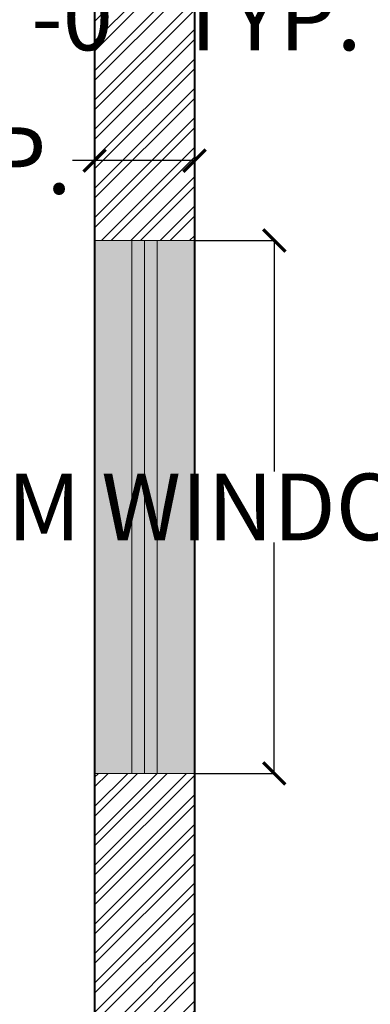
# Model space of a CAD drawing. Units: inches. Extents: x 528 to 2520, y -151 to 1354.
# Tile 25 of 41: x 1407 to 1439, y 1151 to 1239. Entities that reach past the tile are written whole.
import ezdxf

# ---------------------------------------------------------------- set-up
doc = ezdxf.new("R2010")
doc.units = ezdxf.units.IN
doc.header["$MEASUREMENT"] = 0
for name, color, linetype, lineweight in [('A-ANNO-DIMS', 2, 'Continuous', 18), ('A-WALL-PATT', 6, 'Continuous', 13), ('walls', 7, 'Continuous', 40), ('WINDOWS', 2, 'Continuous', 20)]:
    doc.layers.add(name, color=color, linetype=linetype, lineweight=lineweight)
doc.layers.add('A-GLAZ-PATT', color=152, linetype='Continuous', lineweight=13, true_color=0x2776bb)
doc.styles.get("Standard").update_dxf_attribs({"font": 'arial.ttf'})
doc.dimstyles.get("Standard").update_dxf_attribs({"dimtxt": 6, "dimasz": 2, "dimexe": 0.18, "dimexo": 0.0625, "dimgap": 0.09, "dimtad": 0, "dimtih": 1, "dimtoh": 1, "dimdec": 1, "dimzin": 0, "dimdsep": 46, "dimlunit": 3, "dimtxsty": 'Standard', "dimblk": 'ARCHTICK', "dimcen": 0.09, "dimadec": 0, "dimazin": 0, "dimtfac": 1, "dimtdec": 1, "dimtofl": 0, "dimtmove": 0, "dimatfit": 3, "dimfxl": 1, "dimtolj": 1, "dimtzin": 0, "dimarcsym": 0})

# ---------------------------------------------------------------- blocks, each defined once
blk = doc.blocks.new('_ArchTick')
at = {"color": 0, "linetype": 'ByBlock', "const_width": 0.15}
blk.add_lwpolyline([(-0.5, -0.5), (0.5, 0.5)], dxfattribs=at)
blk = doc.blocks.new('*D26')
at = {"layer": 'A-ANNO-DIMS', "color": 0, "lineweight": -2, "transparency": 16777216}
for p, q in [((1422.946, 1317.103), (1446.405, 1317.103)), ((1446.225, 1317.103), (1446.225, 1069.756)), ((1446.225, 816.103), (1446.225, 1063.449)), ((1422.946, 816.103), (1446.405, 816.103))]:
    blk.add_line(p, q, dxfattribs=at)
at = {"layer": 'Defpoints', "color": 0, "transparency": 16777216}
for p in [(1422.883, 1317.103), (1422.883, 816.103), (1446.225, 816.103)]:
    blk.add_point(p, dxfattribs=at)
at = {"layer": 'A-ANNO-DIMS', "color": 0, "lineweight": -2, "transparency": 16777216, "xscale": 2, "yscale": 2, "zscale": 2}
for p, rotation in [((1446.225, 1317.103), 90), ((1446.225, 816.103), 270)]:
    blk.add_blockref('_ArchTick', p, dxfattribs=dict(at, rotation=rotation))
at = {"layer": 'A-ANNO-DIMS', "color": 0, "transparency": 16777216, "insert": (1446.225, 1066.603), "char_height": 6, "attachment_point": 5}
blk.add_mtext('\\A1;41\'-9.0"', dxfattribs=at)
blk = doc.blocks.new('WINDOW-48x9-PLAN')
for p, q in [((0, 5.632), (48, 5.632)), ((0, 4.5), (48, 4.5)), ((0, 3.368), (48, 3.368))]:
    blk.add_line(p, q)
blk.add_lwpolyline([(0, 9), (48, 9), (48, 0), (0, 0)], close=True)
blk = doc.blocks.new('*D44')
at = {"layer": 'A-ANNO-DIMS', "color": 0, "lineweight": -2, "transparency": 16777216}
for p, q in [((1422.946, 1219.369), (1430.263, 1219.369)), ((1430.083, 1219.369), (1430.083, 1198.563)), ((1430.083, 1171.369), (1430.083, 1192.174)), ((1422.946, 1171.369), (1430.263, 1171.369))]:
    blk.add_line(p, q, dxfattribs=at)
at = {"layer": 'Defpoints', "color": 0, "transparency": 16777216}
for p in [(1422.883, 1219.369), (1430.083, 1219.369), (1422.883, 1171.369)]:
    blk.add_point(p, dxfattribs=at)
at = {"layer": 'A-ANNO-DIMS', "color": 0, "lineweight": -2, "transparency": 16777216, "xscale": 2, "yscale": 2, "zscale": 2}
for p, rotation in [((1430.083, 1219.369), 90), ((1430.083, 1171.369), 270)]:
    blk.add_blockref('_ArchTick', p, dxfattribs=dict(at, rotation=rotation))
at = {"layer": 'A-ANNO-DIMS', "color": 0, "transparency": 16777216, "insert": (1430.083, 1195.369), "char_height": 6, "attachment_point": 5}
blk.add_mtext('\\A1;BEDROOM WINDOW 4\'-0" TYP.', dxfattribs=at)
blk = doc.blocks.new('*D45')
at = {"layer": 'A-ANNO-DIMS', "color": 0, "lineweight": -2, "transparency": 16777216}
for p, q in [((1413.883, 1219.431), (1413.883, 1226.749)), ((1422.883, 1219.431), (1422.883, 1226.749)), ((1413.883, 1226.569), (1411.883, 1226.569)), ((1422.883, 1226.569), (1413.883, 1226.569))]:
    blk.add_line(p, q, dxfattribs=at)
at = {"layer": 'Defpoints', "color": 0, "transparency": 16777216}
for p in [(1413.883, 1226.569), (1413.883, 1219.369), (1422.883, 1219.369)]:
    blk.add_point(p, dxfattribs=at)
at = {"layer": 'A-ANNO-DIMS', "color": 0, "lineweight": -2, "transparency": 16777216, "xscale": 2, "yscale": 2, "zscale": 2, "rotation": 180}
blk.add_blockref('_ArchTick', (1413.883, 1226.569), dxfattribs=at)
at = {"layer": 'A-ANNO-DIMS', "color": 0, "lineweight": -2, "transparency": 16777216, "xscale": 2, "yscale": 2, "zscale": 2}
blk.add_blockref('_ArchTick', (1422.883, 1226.569), dxfattribs=at)
at = {"layer": 'A-ANNO-DIMS', "color": 0, "transparency": 16777216, "insert": (1393.507, 1226.569), "char_height": 6, "attachment_point": 5}
blk.add_mtext('\\A1;0\'-9" TYP.', dxfattribs=at)
blk = doc.blocks.new('*D86')
at = {"layer": 'A-ANNO-DIMS', "color": 0, "lineweight": -2, "transparency": 16777216}
for p, q in [((1297.45, 1243.04), (1297.45, 1239.323)), ((1321.45, 1243.04), (1321.45, 1239.323)), ((1297.45, 1239.503), (1321.45, 1239.503)), ((1321.45, 1239.503), (1323.45, 1239.503))]:
    blk.add_line(p, q, dxfattribs=at)
at = {"layer": 'Defpoints', "color": 0, "transparency": 16777216}
for p in [(1297.45, 1243.103), (1321.45, 1243.103), (1321.45, 1239.503)]:
    blk.add_point(p, dxfattribs=at)
at = {"layer": 'A-ANNO-DIMS', "color": 0, "lineweight": -2, "transparency": 16777216, "xscale": 2, "yscale": 2, "zscale": 2, "rotation": 180}
blk.add_blockref('_ArchTick', (1297.45, 1239.503), dxfattribs=at)
at = {"layer": 'A-ANNO-DIMS', "color": 0, "lineweight": -2, "transparency": 16777216, "xscale": 2, "yscale": 2, "zscale": 2}
blk.add_blockref('_ArchTick', (1321.45, 1239.503), dxfattribs=at)
at = {"layer": 'A-ANNO-DIMS', "color": 0, "transparency": 16777216, "insert": (1382.441, 1239.503), "char_height": 6, "attachment_point": 5}
blk.add_mtext('\\A1;BALCONY WINDOW 2\'-0" TYP.', dxfattribs=at)

msp = doc.modelspace()

# ---------------------------------------------------------------- hatches: boundary and pattern name
at = {"layer": 'A-GLAZ-PATT'}
h = msp.add_hatch(color=256, dxfattribs=at)
h.dxf.hatch_style = 1
h.paths.add_polyline_path([(1413.883, 1219.369), (1413.883, 1171.369), (1417.252, 1171.369), (1417.252, 1219.369)])
h.paths.add_polyline_path([(1417.252, 1219.369), (1417.252, 1171.369), (1418.383, 1171.369), (1418.383, 1219.369)])
h.paths.add_polyline_path([(1418.383, 1219.369), (1418.383, 1171.369), (1419.515, 1171.369), (1419.515, 1219.369)])
h.paths.add_polyline_path([(1419.515, 1219.369), (1419.515, 1171.369), (1422.883, 1171.369), (1422.883, 1219.369)])
at = {"layer": 'A-WALL-PATT'}
h = msp.add_hatch(dxfattribs=at)
h.set_pattern_fill('ANSI32', color=256, scale=5)
h.set_pattern_definition([(45, (537.1868, 0), (-1.3258252, 1.3258252), []), (45, (538.0707, 0), (-1.3258252, 1.3258252), [])])
h.paths.add_polyline_path([(1132.883, 1163.855), (1123.883, 1163.855), (1123.883, 969.103), (1135.43, 969.103), (1140.43, 969.103), (1140.43, 974.103), (1132.883, 974.103), (1132.883, 1082.103), (1228.883, 1082.103), (1228.883, 1087.103), (1228.883, 1106.103), (1234.883, 1106.103), (1234.883, 1111.103), (1223.883, 1111.103), (1223.883, 1087.103), (1132.883, 1087.103)])
h.paths.add_polyline_path([(1225.889, 974.103), (1188.43, 974.103), (1188.43, 969.103), (1225.889, 969.103)])
h.paths.add_polyline_path([(1422.883, 1171.369), (1413.883, 1171.369), (1413.883, 1111.103), (1323.883, 1111.103), (1323.883, 1106.103), (1413.883, 1106.103), (1413.883, 974.103), (1323.883, 974.103), (1323.883, 969.103), (1413.883, 969.103), (1413.883, 825.103), (1371.883, 825.103), (1371.883, 816.103), (1422.883, 816.103)])
h.paths.add_polyline_path([(1422.883, 1317.103), (1413.839, 1317.103), (1413.839, 1308.103), (1413.883, 1308.103), (1413.883, 1248.103), (1359.883, 1248.103), (1359.883, 1243.103), (1413.883, 1243.103), (1413.883, 1219.369), (1422.883, 1219.369)])
h.paths.add_polyline_path([(1389.839, 1317.103), (1324.883, 1317.103), (1324.883, 1248.103), (1321.45, 1248.103), (1321.45, 1243.103), (1329.883, 1243.103), (1329.883, 1249.103), (1329.883, 1308.103), (1389.839, 1308.103)])
h.paths.add_polyline_path([(1221.883, 1317.103), (1156.883, 1317.103), (1156.883, 1308.103), (1216.883, 1308.103), (1216.883, 1248.103), (1216.883, 1243.103), (1221.883, 1243.103), (1221.883, 1248.248)])
h.paths.add_polyline_path([(1132.883, 1308.103), (1132.883, 1317.103), (1123.883, 1317.103), (1123.883, 1211.855), (1132.883, 1211.855), (1132.883, 1243.103), (1186.883, 1243.103), (1186.883, 1248.103), (1132.883, 1248.103)])
h.paths.add_polyline_path([(1281.883, 969.103), (1281.883, 974.103), (1261.889, 974.103), (1261.889, 969.103), (1276.883, 969.103), (1276.883, 874.287), (1281.883, 874.287)])
h.paths.add_polyline_path([(1276.883, 969.103), (1264.883, 969.103), (1264.883, 965.117), (1267.922, 965.117), (1267.922, 961.676), (1271.621, 961.676), (1271.621, 957.24), (1276.883, 957.24)], flags=17)
h.paths.add_polyline_path([(1323.883, 825.103), (1281.883, 825.103), (1281.883, 832.287), (1276.883, 832.287), (1276.883, 816.103), (1323.883, 816.103)])

# ---------------------------------------------------------------- linework, layer by layer
at = {"layer": 'walls'}
for p, q in [((1422.883, 1317.103), (1422.883, 816.103)), ((1413.883, 1243.103), (1413.883, 1111.103))]:
    msp.add_line(p, q, dxfattribs=at)

# ---------------------------------------------------------------- block references
at = {"layer": 'WINDOWS', "rotation": 90.00000000000006}
msp.add_blockref('WINDOW-48x9-PLAN', (1422.883, 1171.369), dxfattribs=at)

# ---------------------------------------------------------------- dimensions: what is measured, and where the dimension line sits
at = {"layer": 'A-ANNO-DIMS'}
dim = msp.add_linear_dim(base=(1446.225, 816.103), p1=(1422.883, 1317.103), p2=(1422.883, 816.103), angle=90, dimstyle='Standard', override={"dimclrd": 0, "dimclre": 0, "dimclrt": 0}, dxfattribs=at)
dim.commit()
dim.dimension.update_dxf_attribs({"geometry": '*D26', "text_midpoint": (1446.225, 1066.603)})
dim = msp.add_linear_dim(base=(1321.45, 1239.503), p1=(1297.45, 1243.103), p2=(1321.45, 1243.103), text='BALCONY WINDOW <> TYP.', dimstyle='Standard', override={"dimdec": 1, "dimlfac": 1, "dimrnd": 0, "dimzin": 1, "dimdsep": 46, "dimlunit": 4, "dimfrac": 2}, dxfattribs=at)
dim.commit()
dim.dimension.update_dxf_attribs({"geometry": '*D86', "text_midpoint": (1382.441, 1239.503)})
for base, p1, p2, angle, text, picture, middle in [((1413.883, 1226.569), (1422.883, 1219.369), (1413.883, 1219.369), 180, '<> TYP.', '*D45', (1393.507, 1226.569)), ((1430.083, 1219.369), (1422.883, 1171.369), (1422.883, 1219.369), 90, 'BEDROOM WINDOW <> TYP.', '*D44', (1430.083, 1195.369))]:
    dim = msp.add_linear_dim(base=base, p1=p1, p2=p2, angle=angle, text=text, dimstyle='Standard', override={"dimdec": 1, "dimlfac": 1, "dimrnd": 0, "dimzin": 1, "dimdsep": 46, "dimlunit": 4, "dimfrac": 2}, dxfattribs=at)
    dim.commit()
    dim.dimension.update_dxf_attribs({"geometry": picture, "text_midpoint": middle})

doc.saveas('drawing.dxf')
